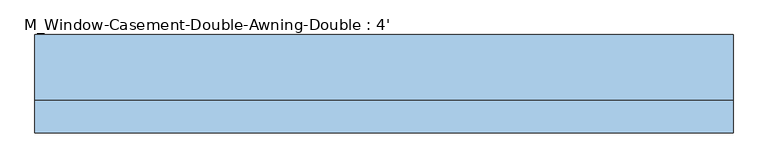
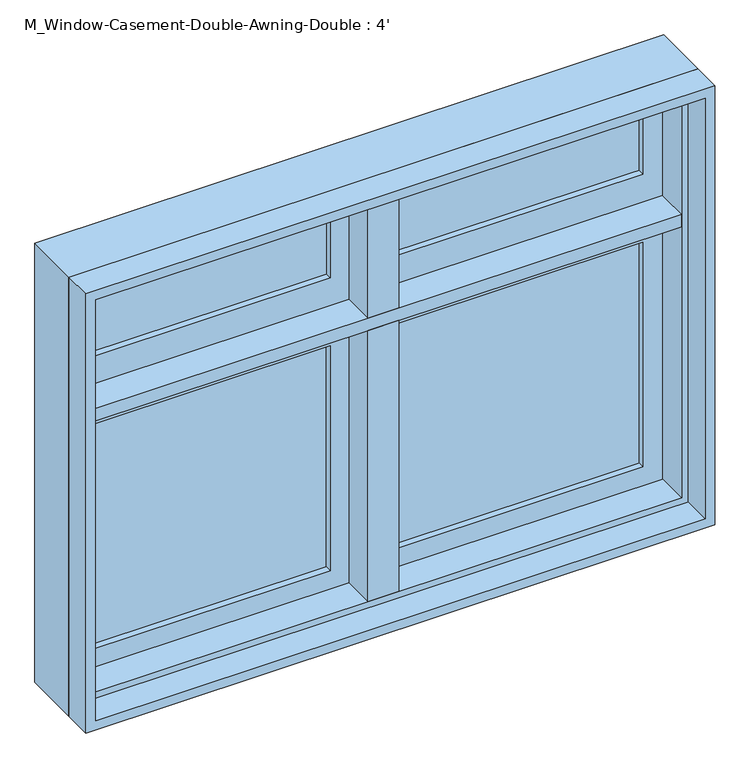
"""IFC4 building model written with IfcOpenShell, lengths in millimetres: window geometry, M_Window-Casement-Double-Awning-Double : 4'."""

from ifc_helpers import new_model, si_unit, frame, origin, place, context, project, spatial, polyline, outline, extrude, faceted_brep, source, transform, mapped, element, save


def m_window_casement_double_awning_double_4_7efa9bbd(model_context):
    return source(origin(), model_context, "Body", "SolidModel", [
        faceted_brep([(577.85, 44.45, 1768.25), (577.85, -19.05, 1768.25), (-577.85, -19.05, 1768.25), (-577.85, 44.45, 1768.25), (596.9, 95.25, 1787.3), (596.9, 44.45, 1787.3), (-596.9, 44.45, 1787.3), (-596.9, 95.25, 1787.3), (609.6, -19.05, 1800.0), (609.6, 95.25, 1800.0), (-609.6, 95.25, 1800.0), (-609.6, -19.05, 1800.0), (-577.85, -19.05, 931.75), (-577.85, 44.45, 931.75), (-596.9, 44.45, 912.7), (-596.9, 95.25, 912.7), (-609.6, 95.25, 900.0), (-609.6, -19.05, 900.0), (577.85, -19.05, 931.75), (577.85, 44.45, 931.75), (596.9, 44.45, 912.7), (596.9, 95.25, 912.7), (609.6, 95.25, 900.0), (609.6, -19.05, 900.0)], [[[0, 1, 2, 3]], [[4, 5, 6, 7]], [[8, 9, 10, 11]], [[3, 2, 12, 13]], [[7, 6, 14, 15]], [[11, 10, 16, 17]], [[13, 12, 18, 19]], [[15, 14, 20, 21]], [[17, 16, 22, 23]], [[11, 17, 23, 8], [1, 18, 12, 2]], [[19, 18, 1, 0]], [[5, 20, 14, 6], [3, 13, 19, 0]], [[21, 20, 5, 4]], [[23, 22, 9, 8]], [[9, 22, 16, 10], [7, 15, 21, 4]]]),
        extrude(outline(polyline([(1800.0, -609.6), (900.0, -609.6), (900.0, 609.6), (1800.0, 609.6), (1800.0, -609.6)]), holes=[polyline([(1780.95, 590.55), (919.05, 590.55), (919.05, -590.55), (1780.95, -590.55), (1780.95, 590.55)])]), frame((0.0, -76.2, 0.0), z_axis=(0.0, 1.0, 0.0), x_axis=(0.0, 0.0, 1.0)), (0.0, 0.0, 1.0), 57.15),
        extrude(outline(polyline([(912.7, 596.9), (1487.3, 596.9), (1487.3, 9.525), (912.7, 9.525), (912.7, 596.9)]), holes=[polyline([(969.85, 66.675), (1430.15, 66.675), (1430.15, 539.75), (969.85, 539.75), (969.85, 66.675)])]), frame((0.0, 44.45, 0.0), z_axis=(0.0, 1.0, 0.0), x_axis=(0.0, 0.0, 1.0)), (0.0, 0.0, 1.0), 44.45),
        extrude(outline(polyline([(1487.3, -596.9), (912.7, -596.9), (912.7, -9.525), (1487.3, -9.525), (1487.3, -596.9)]), holes=[polyline([(1430.15, -66.675), (969.85, -66.675), (969.85, -539.75), (1430.15, -539.75), (1430.15, -66.675)])]), frame((0.0, 44.45, 0.0), z_axis=(0.0, 1.0, 0.0), x_axis=(0.0, 0.0, 1.0)), (0.0, 0.0, 1.0), 44.45),
        extrude(outline(polyline([(539.75, 76.2), (539.75, 69.85), (66.675, 69.85), (66.675, 76.2), (539.75, 76.2)])), frame((0.0, 0.0, 969.85), z_axis=(0.0, 0.0, 1.0), x_axis=(1.0, 0.0, 0.0)), (0.0, 0.0, 1.0), 460.3),
        extrude(outline(polyline([(66.675, 57.15), (66.675, 63.5), (539.75, 63.5), (539.75, 57.15), (66.675, 57.15)])), frame((0.0, 0.0, 969.85), z_axis=(0.0, 0.0, 1.0), x_axis=(1.0, 0.0, 0.0)), (0.0, 0.0, 1.0), 460.3),
        extrude(outline(polyline([(-66.675, 76.2), (-66.675, 69.85), (-539.75, 69.85), (-539.75, 76.2), (-66.675, 76.2)])), frame((0.0, 0.0, 969.85), z_axis=(0.0, 0.0, 1.0), x_axis=(1.0, 0.0, 0.0)), (0.0, 0.0, 1.0), 460.3),
        extrude(outline(polyline([(-539.75, 57.15), (-539.75, 63.5), (-66.675, 63.5), (-66.675, 57.15), (-539.75, 57.15)])), frame((0.0, 0.0, 969.85), z_axis=(0.0, 0.0, 1.0), x_axis=(1.0, 0.0, 0.0)), (0.0, 0.0, 1.0), 460.3),
        faceted_brep([(9.525, 95.25, 1487.3), (-9.525, 95.25, 1487.3), (-9.525, 44.45, 1487.3), (-30.1625, 44.45, 1487.3), (-30.1625, -19.05, 1487.3), (30.1625, -19.05, 1487.3), (30.1625, 44.45, 1487.3), (9.525, 44.45, 1487.3), (9.525, 95.25, 912.7), (9.525, 44.45, 912.7), (-9.525, 44.45, 912.7), (-9.525, 95.25, 912.7), (-9.525, 44.45, 931.75), (-30.1625, 44.45, 931.75), (-30.1625, -19.05, 931.75), (30.1625, -19.05, 931.75), (30.1625, 44.45, 931.75), (9.525, 44.45, 931.75)], [[[0, 1, 2, 3, 4, 5, 6, 7]], [[8, 9, 10, 11]], [[1, 0, 8, 11]], [[2, 1, 11, 10, 12]], [[3, 2, 12, 13]], [[4, 3, 13, 14]], [[5, 4, 14, 15]], [[6, 5, 15, 16]], [[7, 6, 16, 17]], [[0, 7, 17, 9, 8]], [[17, 12, 10, 9]], [[12, 17, 16, 15, 14, 13]]]),
        extrude(outline(polyline([(-66.675, 76.2), (-66.675, 69.85), (-539.75, 69.85), (-539.75, 76.2), (-66.675, 76.2)])), frame((0.0, 0.0, 1569.85), z_axis=(0.0, 0.0, 1.0), x_axis=(1.0, 0.0, 0.0)), (0.0, 0.0, 1.0), 160.3),
        extrude(outline(polyline([(-539.75, 57.15), (-539.75, 63.5), (-66.675, 63.5), (-66.675, 57.15), (-539.75, 57.15)])), frame((0.0, 0.0, 1569.85), z_axis=(0.0, 0.0, 1.0), x_axis=(1.0, 0.0, 0.0)), (0.0, 0.0, 1.0), 160.3),
        extrude(outline(polyline([(596.9, 95.25), (596.9, 44.45), (577.85, 44.45), (577.85, -19.05), (-577.85, -19.05), (-577.85, 44.45), (-596.9, 44.45), (-596.9, 95.25), (596.9, 95.25)])), frame((0.0, 0.0, 1487.3), z_axis=(0.0, 0.0, 1.0), x_axis=(1.0, 0.0, 0.0)), (0.0, 0.0, 1.0), 25.4),
        faceted_brep([(9.525, 44.45, 1787.3), (9.525, 95.25, 1787.3), (-9.525, 95.25, 1787.3), (-9.525, 44.45, 1787.3), (-9.525, 44.45, 1512.7), (-9.525, 95.25, 1512.7), (9.525, 95.25, 1512.7), (9.525, 44.45, 1512.7), (30.1625, 44.45, 1512.7), (30.1625, -19.05, 1512.7), (-30.1625, -19.05, 1512.7), (-30.1625, 44.45, 1512.7), (-30.1625, 44.45, 1768.25), (-9.525, 44.45, 1768.25), (-30.1625, -19.05, 1768.25), (30.1625, -19.05, 1768.25), (30.1625, 44.45, 1768.25), (9.525, 44.45, 1768.25)], [[[0, 1, 2, 3]], [[4, 5, 6, 7, 8, 9, 10, 11]], [[4, 11, 12, 13]], [[11, 10, 14, 12]], [[10, 9, 15, 14]], [[9, 8, 16, 15]], [[8, 7, 17, 16]], [[1, 0, 17, 7, 6]], [[2, 1, 6, 5]], [[3, 2, 5, 4, 13]], [[17, 13, 12, 14, 15, 16]], [[13, 17, 0, 3]]]),
        extrude(outline(polyline([(1787.3, 9.525), (1512.7, 9.525), (1512.7, 596.9), (1787.3, 596.9), (1787.3, 9.525)]), holes=[polyline([(1730.15, 539.75), (1569.85, 539.75), (1569.85, 66.675), (1730.15, 66.675), (1730.15, 539.75)])]), frame((0.0, 44.45, 0.0), z_axis=(0.0, 1.0, 0.0), x_axis=(0.0, 0.0, 1.0)), (0.0, 0.0, 1.0), 44.45),
        extrude(outline(polyline([(1512.7, -9.525), (1787.3, -9.525), (1787.3, -596.9), (1512.7, -596.9), (1512.7, -9.525)]), holes=[polyline([(1569.85, -539.75), (1730.15, -539.75), (1730.15, -66.675), (1569.85, -66.675), (1569.85, -539.75)])]), frame((0.0, 44.45, 0.0), z_axis=(0.0, 1.0, 0.0), x_axis=(0.0, 0.0, 1.0)), (0.0, 0.0, 1.0), 44.45),
        extrude(outline(polyline([(66.675, 76.2), (539.75, 76.2), (539.75, 69.85), (66.675, 69.85), (66.675, 76.2)])), frame((0.0, 0.0, 1569.85), z_axis=(0.0, 0.0, 1.0), x_axis=(1.0, 0.0, 0.0)), (0.0, 0.0, 1.0), 160.3),
        extrude(outline(polyline([(539.75, 57.15), (66.675, 57.15), (66.675, 63.5), (539.75, 63.5), (539.75, 57.15)])), frame((0.0, 0.0, 1569.85), z_axis=(0.0, 0.0, 1.0), x_axis=(1.0, 0.0, 0.0)), (0.0, 0.0, 1.0), 160.3),
    ])


if __name__ == "__main__":
    model = new_model("IFC4")
    model_context = context("Model", 3, world=origin())
    ifc_project = project(units=[si_unit("LENGTHUNIT", "METRE", prefix="MILLI")], contexts=[model_context])
    site = spatial("IfcSite", under=ifc_project)
    building = spatial("IfcBuilding", under=site)
    placement = place(None, origin())
    m_window_casement_double_awning_double_4_shape = m_window_casement_double_awning_double_4_7efa9bbd(model_context)
    element("IfcWindow", 1, ObjectType="M_Window-Casement-Double-Awning-Double : 4'", at=placement, inside=building, context=model_context, shape_type="MappedRepresentation", body=[
        mapped(m_window_casement_double_awning_double_4_shape, transform((0.0, 0.0, 0.0), x_axis=(1.0, 0.0, 0.0), y_axis=(0.0, 1.0, 0.0), z_axis=(0.0, 0.0, 1.0))),
    ])
    save(model, "model.ifc")

# Revit data of these elements
# Type "M_Window-Casement-Double-Awning-Double : 4'"
#   Type Mark = "11"
#   Fire Rating = "0.5h"
#   Assembly Code = "B2020100"
#   Analytic Construction = "Double glazing - domestic"
#   Window Inset [instance default] = 0' - 0"
#   Wall Thickness [instance default] = 0' - 5.90551"
#   Interior Wall Closure [instance default] = 0' - 2.15551"
#   Half Width = 2' - 0"
#   Visual Light Transmittance = 0.81
#   Transom Height = 0' - 11.81102"
#   Thermal Resistance (R) = 1.8146 (h·ft²·°F)/BTU
#   Solar Heat Gain Coefficient = 0.76
#   Rough Width = 4' - 0.59055"
#   Rough Height = 3' - 0.02362"
#   Open Window Height = 1' - 11.62205"
#   Frame Extension [instance default] = 0' - 0 1/4"
#   Height = 2' - 11.43307"
#   Heat Transfer Coefficient (U) = 0.5511 BTU/(h·ft²·°F)
#   Exterior Wall Closure [instance default] = 0' - 1.25197"
#   Extension Jamb [instance default] = 0' - 2.15551"
#   Default Sill Height = 2' - 11.43307"
#   Width = 4' - 0"
#   Top Muntin Visibility = yes
#   Bottom Muntin Visibility = yes
#   Interior Trim Visibility [instance default] = yes
#   Exterior Trim Visibility [instance default] = yes
#   Extension Jamb Visibility [instance default] = yes
#   Interior Trim Material = Wood - Stained
#   Muntin Pattern = M_Muntin Pattern_2x2 : M_Muntin Pattern_2x2
#   Interior Trim = M_Trim-Window-Interior-Flat : Picture Frame
#   Interior Frame Material = Wood - Stained
#   Glass Panel Material = Glass
#   Exterior Trim Material = Clad - White
#   Exterior Trim = M_Trim-Window-Exterior-Flat : with Sill
#   Exterior Frame Material = Clad - White
#   Wall Closure = (empty or 0)
# Element 1 (IfcWindow, "M_Window-Casement-Double-Awning-Double : 4'")
#   Wall Thickness = 0' - 6"
#   Extension Jamb = 0' - 2 1/4"
#   Materials on its faces: "Wood - Stained", "Glass", "Clad - White"
# Materials
#   "Wood - Stained": class "Wood", colour RGB 227 170 128, transparency 0, Cost = 0
#   "Glass": class "Glass", colour RGB 218 227 224, transparency 0.85, Description = "Soda Lime Glass", Cost = 0
#   "Clad - White": class "Wood", colour RGB 242 242 238, transparency 0, Cost = 0
